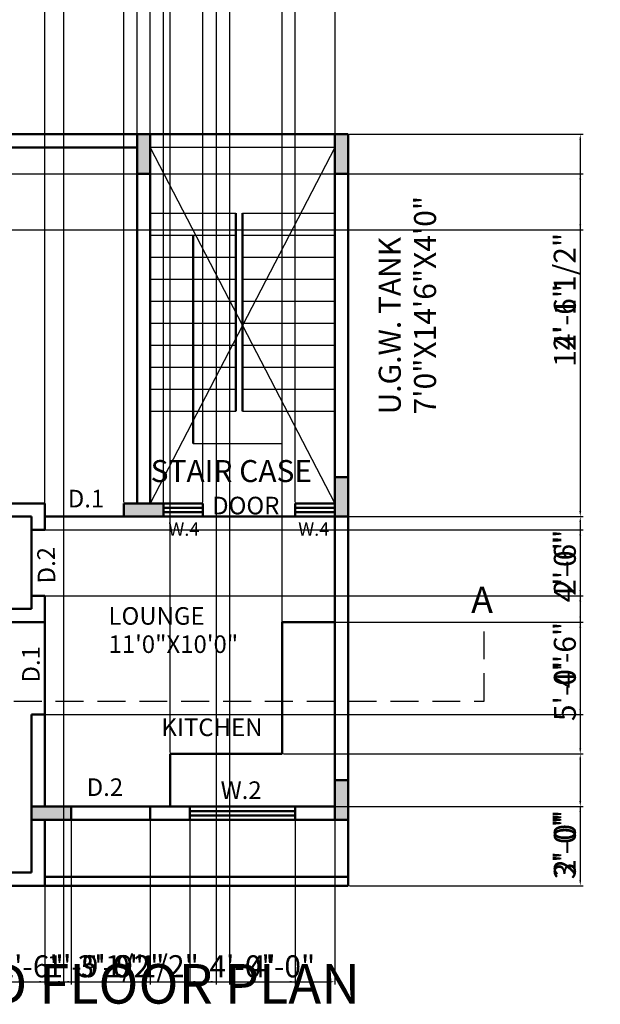
# Model space of a CAD drawing. Units: inches. Extents: x 2368 to 3882, y 1243 to 2139.
# Tile 2 of 6: x 2595 to 2859, y 1243 to 1691. Entities that reach past the tile are written whole.
import ezdxf

# ---------------------------------------------------------------- set-up
doc = ezdxf.new("R2010")
doc.units = ezdxf.units.IN
doc.linetypes.add('DASHED', pattern=[19.05, 12.7, -6.35])
for name, color, linetype, lineweight in [('A-ANNO-DIMS', 2, 'Continuous', 18), ('A-ANNO-SYMB', 1, 'DASHED', 25), ('A-ANNO-TEXT', 7, 'Continuous', 18), ('A-AREA-IDEN', 3, 'Continuous', 18), ('A-FLOR-STRS', 3, 'Continuous', 25), ('A-WALL', 7, 'Continuous', 50), ('A-WALL-PATT', 8, 'Continuous', 13)]:
    doc.layers.add(name, color=color, linetype=linetype, lineweight=lineweight)
doc.styles.get("Standard").update_dxf_attribs({"font": 'arial.ttf'})
doc.dimstyles.new('ISO-25', dxfattribs={"dimtxt": 10, "dimasz": 2.5, "dimexe": 1.25, "dimexo": 0.625, "dimtad": 1, "dimlunit": 3, "dimtxsty": 'Standard', "dimcen": 2.5, "dimadec": 0, "dimazin": 0, "dimtfac": 1, "dimtmove": 0, "dimatfit": 3, "dimfxl": 1, "dimarcsym": 0})

# ---------------------------------------------------------------- blocks, each defined once
blk = doc.blocks.new('*D35')
at = {"layer": 'A-ANNO-DIMS', "color": 0, "lineweight": -2, "transparency": 16777216}
for p, q in [((2585.04, 1776.18), (2585.04, 1251.93)), ((2615.04, 1776.18), (2615.04, 1251.93)), ((2587.54, 1253.18), (2612.54, 1253.18))]:
    blk.add_line(p, q, dxfattribs=at)
at = {"layer": 'A-ANNO-DIMS', "color": 0, "transparency": 16777216}
for points in [[(2587.54, 1253.6), (2587.54, 1252.77), (2585.04, 1253.18)], [(2612.54, 1253.6), (2612.54, 1252.77), (2615.04, 1253.18)]]:
    blk.add_solid(points, dxfattribs=at)
at = {"layer": 'Defpoints', "color": 0, "transparency": 16777216}
for p in [(2585.04, 1776.81), (2615.04, 1776.81), (2615.04, 1253.18)]:
    blk.add_point(p, dxfattribs=at)
at = {"layer": 'A-ANNO-DIMS', "color": 0, "transparency": 16777216, "insert": (2600.04, 1258.91), "char_height": 10, "attachment_point": 5}
blk.add_mtext('2\'-6"', dxfattribs=at)
blk = doc.blocks.new('*D36')
at = {"layer": 'A-ANNO-DIMS', "color": 0, "lineweight": -2, "transparency": 16777216}
for p, q in [((2615.04, 1776.18), (2615.04, 1251.93)), ((2684.5, 1770.18), (2684.5, 1251.93)), ((2617.54, 1253.18), (2682, 1253.18))]:
    blk.add_line(p, q, dxfattribs=at)
at = {"layer": 'A-ANNO-DIMS', "color": 0, "transparency": 16777216}
for points in [[(2617.54, 1253.6), (2617.54, 1252.77), (2615.04, 1253.18)], [(2682, 1253.6), (2682, 1252.77), (2684.5, 1253.18)]]:
    blk.add_solid(points, dxfattribs=at)
at = {"layer": 'Defpoints', "color": 0, "transparency": 16777216}
for p in [(2615.04, 1776.81), (2684.5, 1770.81), (2684.5, 1253.18)]:
    blk.add_point(p, dxfattribs=at)
at = {"layer": 'A-ANNO-DIMS', "color": 0, "transparency": 16777216, "insert": (2649.77, 1258.98), "char_height": 10, "attachment_point": 5}
blk.add_mtext('5\'-9 1/2"', dxfattribs=at)
blk = doc.blocks.new('*D37')
at = {"layer": 'A-ANNO-DIMS', "color": 0, "lineweight": -2, "transparency": 16777216}
for p, q in [((2690.5, 1770.18), (2690.5, 1251.93)), ((2738.5, 1770.18), (2738.5, 1251.93)), ((2693, 1253.18), (2736, 1253.18))]:
    blk.add_line(p, q, dxfattribs=at)
at = {"layer": 'A-ANNO-DIMS', "color": 0, "transparency": 16777216}
for points in [[(2693, 1253.6), (2693, 1252.77), (2690.5, 1253.18)], [(2736, 1253.6), (2736, 1252.77), (2738.5, 1253.18)]]:
    blk.add_solid(points, dxfattribs=at)
at = {"layer": 'Defpoints', "color": 0, "transparency": 16777216}
for p in [(2690.5, 1770.81), (2738.5, 1770.81), (2738.5, 1253.18)]:
    blk.add_point(p, dxfattribs=at)
at = {"layer": 'A-ANNO-DIMS', "color": 0, "transparency": 16777216, "insert": (2714.5, 1258.91), "char_height": 10, "attachment_point": 5}
blk.add_mtext('4\'-0"', dxfattribs=at)
blk = doc.blocks.new('*D45')
at = {"layer": 'A-ANNO-DIMS', "color": 0, "lineweight": -2, "transparency": 16777216}
for p, q in [((2745.12, 1638.88), (2851.45, 1638.88)), ((2850.2, 1636.38), (2850.2, 1467.38)), ((2739.12, 1464.88), (2851.45, 1464.88))]:
    blk.add_line(p, q, dxfattribs=at)
at = {"layer": 'A-ANNO-DIMS', "color": 0, "transparency": 16777216}
for points in [[(2849.79, 1636.38), (2850.62, 1636.38), (2850.2, 1638.88)], [(2849.79, 1467.38), (2850.62, 1467.38), (2850.2, 1464.88)]]:
    blk.add_solid(points, dxfattribs=at)
at = {"layer": 'Defpoints', "color": 0, "transparency": 16777216}
for p in [(2744.5, 1638.88), (2738.5, 1464.88), (2850.2, 1464.88)]:
    blk.add_point(p, dxfattribs=at)
at = {"layer": 'A-ANNO-DIMS', "color": 0, "transparency": 16777216, "insert": (2844.47, 1551.88), "char_height": 10, "attachment_point": 5, "rotation": 90}
blk.add_mtext('14\'-6"', dxfattribs=at)
blk = doc.blocks.new('*D46')
at = {"layer": 'A-ANNO-DIMS', "color": 0, "lineweight": -2, "transparency": 16777216}
for p, q in [((2739.12, 1464.88), (2851.45, 1464.88)), ((2850.2, 1462.38), (2850.2, 1419.38)), ((2715.12, 1416.88), (2851.45, 1416.88))]:
    blk.add_line(p, q, dxfattribs=at)
at = {"layer": 'A-ANNO-DIMS', "color": 0, "transparency": 16777216}
for points in [[(2849.79, 1462.38), (2850.62, 1462.38), (2850.2, 1464.88)], [(2849.79, 1419.38), (2850.62, 1419.38), (2850.2, 1416.88)]]:
    blk.add_solid(points, dxfattribs=at)
at = {"layer": 'Defpoints', "color": 0, "transparency": 16777216}
for p in [(2738.5, 1464.88), (2714.5, 1416.88), (2850.2, 1416.88)]:
    blk.add_point(p, dxfattribs=at)
at = {"layer": 'A-ANNO-DIMS', "color": 0, "transparency": 16777216, "insert": (2844.47, 1440.88), "char_height": 10, "attachment_point": 5, "rotation": 90}
blk.add_mtext('4\'-0"', dxfattribs=at)
blk = doc.blocks.new('*D47')
at = {"layer": 'A-ANNO-DIMS', "color": 0, "lineweight": -2, "transparency": 16777216}
for p, q in [((2715.12, 1416.88), (2851.45, 1416.88)), ((2850.2, 1414.38), (2850.2, 1359.38)), ((2715.12, 1356.88), (2851.45, 1356.88))]:
    blk.add_line(p, q, dxfattribs=at)
at = {"layer": 'A-ANNO-DIMS', "color": 0, "transparency": 16777216}
for points in [[(2849.79, 1414.38), (2850.62, 1414.38), (2850.2, 1416.88)], [(2849.79, 1359.38), (2850.62, 1359.38), (2850.2, 1356.88)]]:
    blk.add_solid(points, dxfattribs=at)
at = {"layer": 'Defpoints', "color": 0, "transparency": 16777216}
for p in [(2714.5, 1416.88), (2714.5, 1356.88), (2850.2, 1356.88)]:
    blk.add_point(p, dxfattribs=at)
at = {"layer": 'A-ANNO-DIMS', "color": 0, "transparency": 16777216, "insert": (2844.47, 1386.88), "char_height": 10, "attachment_point": 5, "rotation": 90}
blk.add_mtext('5\'-0"', dxfattribs=at)
blk = doc.blocks.new('*D48')
at = {"layer": 'A-ANNO-DIMS', "color": 0, "lineweight": -2, "transparency": 16777216}
for p, q in [((2715.12, 1356.88), (2851.45, 1356.88)), ((2850.2, 1354.38), (2850.2, 1335.38)), ((2739.12, 1332.88), (2851.45, 1332.88)), ((2850.2, 1332.88), (2850.2, 1302.38))]:
    blk.add_line(p, q, dxfattribs=at)
at = {"layer": 'A-ANNO-DIMS', "color": 0, "transparency": 16777216}
for points in [[(2849.79, 1354.38), (2850.62, 1354.38), (2850.2, 1356.88)], [(2849.79, 1335.38), (2850.62, 1335.38), (2850.2, 1332.88)]]:
    blk.add_solid(points, dxfattribs=at)
at = {"layer": 'Defpoints', "color": 0, "transparency": 16777216}
for p in [(2714.5, 1356.88), (2738.5, 1332.88), (2850.2, 1332.88)]:
    blk.add_point(p, dxfattribs=at)
at = {"layer": 'A-ANNO-DIMS', "color": 0, "transparency": 16777216, "insert": (2844.47, 1316.38), "char_height": 10, "attachment_point": 5, "rotation": 90}
blk.add_mtext('2\'-0"', dxfattribs=at)
blk = doc.blocks.new('*D49')
at = {"layer": 'A-ANNO-DIMS', "color": 0, "lineweight": -2, "transparency": 16777216}
for p, q in [((2739.12, 1332.88), (2851.45, 1332.88)), ((2850.2, 1330.38), (2850.2, 1299.38)), ((2745.12, 1296.88), (2851.45, 1296.88))]:
    blk.add_line(p, q, dxfattribs=at)
at = {"layer": 'A-ANNO-DIMS', "color": 0, "transparency": 16777216}
for points in [[(2849.79, 1330.38), (2850.62, 1330.38), (2850.2, 1332.88)], [(2849.79, 1299.38), (2850.62, 1299.38), (2850.2, 1296.88)]]:
    blk.add_solid(points, dxfattribs=at)
at = {"layer": 'Defpoints', "color": 0, "transparency": 16777216}
for p in [(2738.5, 1332.88), (2744.5, 1296.88), (2850.2, 1296.88)]:
    blk.add_point(p, dxfattribs=at)
at = {"layer": 'A-ANNO-DIMS', "color": 0, "transparency": 16777216, "insert": (2844.47, 1314.88), "char_height": 10, "attachment_point": 5, "rotation": 90}
blk.add_mtext('3\'-0"', dxfattribs=at)
blk = doc.blocks.new('*D50')
at = {"layer": 'A-ANNO-DIMS', "color": 0, "lineweight": -2, "transparency": 16777216}
for p, q in [((2582.5, 1633.51), (2582.5, 2127.76)), ((2585, 2126.51), (2646, 2126.51)), ((2648.5, 1639.51), (2648.5, 2127.76))]:
    blk.add_line(p, q, dxfattribs=at)
at = {"layer": 'A-ANNO-DIMS', "color": 0, "transparency": 16777216}
for points in [[(2585, 2126.93), (2585, 2126.09), (2582.5, 2126.51)], [(2646, 2126.93), (2646, 2126.09), (2648.5, 2126.51)]]:
    blk.add_solid(points, dxfattribs=at)
at = {"layer": 'Defpoints', "color": 0, "transparency": 16777216}
for p in [(2648.5, 2126.51), (2648.5, 1638.88), (2582.5, 1632.88)]:
    blk.add_point(p, dxfattribs=at)
at = {"layer": 'A-ANNO-DIMS', "color": 0, "transparency": 16777216, "insert": (2615.5, 2132.24), "char_height": 10, "attachment_point": 5}
blk.add_mtext('5\'-6"', dxfattribs=at)
blk = doc.blocks.new('*D51')
at = {"layer": 'A-ANNO-DIMS', "color": 0, "lineweight": -2, "transparency": 16777216}
for p, q in [((2646, 2126.51), (2643.5, 2126.51)), ((2648.5, 1639.51), (2648.5, 2127.76)), ((2648.5, 2126.51), (2654.5, 2126.51)), ((2654.5, 1639.51), (2654.5, 2127.76)), ((2657, 2126.51), (2687.33, 2126.51))]:
    blk.add_line(p, q, dxfattribs=at)
at = {"layer": 'A-ANNO-DIMS', "color": 0, "transparency": 16777216}
for points in [[(2646, 2126.93), (2646, 2126.09), (2648.5, 2126.51)], [(2657, 2126.93), (2657, 2126.09), (2654.5, 2126.51)]]:
    blk.add_solid(points, dxfattribs=at)
at = {"layer": 'Defpoints', "color": 0, "transparency": 16777216}
for p in [(2654.5, 2126.51), (2648.5, 1638.88), (2654.5, 1638.88)]:
    blk.add_point(p, dxfattribs=at)
at = {"layer": 'A-ANNO-DIMS', "color": 0, "transparency": 16777216, "insert": (2673.41, 2132.24), "char_height": 10, "attachment_point": 5}
blk.add_mtext('0\'-6"', dxfattribs=at)
blk = doc.blocks.new('*D53')
at = {"layer": 'A-ANNO-DIMS', "color": 0, "lineweight": -2, "transparency": 16777216}
for p, q in [((2663.5, 1357.51), (2663.5, 2127.76)), ((2666, 2126.51), (2712, 2126.51)), ((2714.5, 1357.51), (2714.5, 2127.76))]:
    blk.add_line(p, q, dxfattribs=at)
at = {"layer": 'A-ANNO-DIMS', "color": 0, "transparency": 16777216}
for points in [[(2666, 2126.93), (2666, 2126.09), (2663.5, 2126.51)], [(2712, 2126.93), (2712, 2126.09), (2714.5, 2126.51)]]:
    blk.add_solid(points, dxfattribs=at)
at = {"layer": 'Defpoints', "color": 0, "transparency": 16777216}
for p in [(2714.5, 2126.51), (2663.5, 1356.88), (2714.5, 1356.88)]:
    blk.add_point(p, dxfattribs=at)
at = {"layer": 'A-ANNO-DIMS', "color": 0, "transparency": 16777216, "insert": (2689, 2132.24), "char_height": 10, "attachment_point": 5}
blk.add_mtext('4\'-3"', dxfattribs=at)
blk = doc.blocks.new('*D55')
at = {"layer": 'A-ANNO-DIMS', "color": 0, "lineweight": -2, "transparency": 16777216}
for p, q in [((2585.04, 1296.26), (2585.04, 1251.93)), ((2606.5, 1296.26), (2606.5, 1251.93)), ((2587.54, 1253.18), (2604, 1253.18)), ((2606.5, 1253.18), (2659.19, 1253.18))]:
    blk.add_line(p, q, dxfattribs=at)
at = {"layer": 'A-ANNO-DIMS', "color": 0, "transparency": 16777216}
for points in [[(2587.54, 1253.6), (2587.54, 1252.77), (2585.04, 1253.18)], [(2604, 1253.6), (2604, 1252.77), (2606.5, 1253.18)]]:
    blk.add_solid(points, dxfattribs=at)
at = {"layer": 'Defpoints', "color": 0, "transparency": 16777216}
for p in [(2585.04, 1296.88), (2606.5, 1296.88), (2606.5, 1253.18)]:
    blk.add_point(p, dxfattribs=at)
at = {"layer": 'A-ANNO-DIMS', "color": 0, "transparency": 16777216, "insert": (2634.09, 1258.98), "char_height": 10, "attachment_point": 5}
blk.add_mtext('1\'-9 1/2"', dxfattribs=at)
blk = doc.blocks.new('*D56')
at = {"layer": 'A-ANNO-DIMS', "color": 0, "lineweight": -2, "transparency": 16777216}
for p, q in [((2618.5, 1332.26), (2618.5, 1251.93)), ((2654.5, 1332.26), (2654.5, 1251.93)), ((2621, 1253.18), (2652, 1253.18))]:
    blk.add_line(p, q, dxfattribs=at)
at = {"layer": 'A-ANNO-DIMS', "color": 0, "transparency": 16777216}
for points in [[(2621, 1253.6), (2621, 1252.77), (2618.5, 1253.18)], [(2652, 1253.6), (2652, 1252.77), (2654.5, 1253.18)]]:
    blk.add_solid(points, dxfattribs=at)
at = {"layer": 'Defpoints', "color": 0, "transparency": 16777216}
for p in [(2618.5, 1332.88), (2654.5, 1332.88), (2654.5, 1253.18)]:
    blk.add_point(p, dxfattribs=at)
at = {"layer": 'A-ANNO-DIMS', "color": 0, "transparency": 16777216, "insert": (2636.5, 1258.92), "char_height": 10, "attachment_point": 5}
blk.add_mtext('3\'-0"', dxfattribs=at)
blk = doc.blocks.new('*D57')
at = {"layer": 'A-ANNO-DIMS', "color": 0, "lineweight": -2, "transparency": 16777216}
for p, q in [((2672.5, 1326.26), (2672.5, 1251.93)), ((2720.5, 1326.26), (2720.5, 1251.93)), ((2675, 1253.18), (2718, 1253.18))]:
    blk.add_line(p, q, dxfattribs=at)
at = {"layer": 'A-ANNO-DIMS', "color": 0, "transparency": 16777216}
for points in [[(2675, 1253.6), (2675, 1252.77), (2672.5, 1253.18)], [(2718, 1253.6), (2718, 1252.77), (2720.5, 1253.18)]]:
    blk.add_solid(points, dxfattribs=at)
at = {"layer": 'Defpoints', "color": 0, "transparency": 16777216}
for p in [(2672.5, 1326.88), (2720.5, 1326.88), (2720.5, 1253.18)]:
    blk.add_point(p, dxfattribs=at)
at = {"layer": 'A-ANNO-DIMS', "color": 0, "transparency": 16777216, "insert": (2696.5, 1258.91), "char_height": 10, "attachment_point": 5}
blk.add_mtext('4\'-0"', dxfattribs=at)
blk = doc.blocks.new('*D59')
at = {"layer": 'A-ANNO-DIMS', "color": 0, "lineweight": -2, "transparency": 16777216}
for p, q in [((2606.5, 1465.51), (2606.5, 2127.76)), ((2609, 2126.51), (2640, 2126.51)), ((2642.5, 1471.51), (2642.5, 2127.76))]:
    blk.add_line(p, q, dxfattribs=at)
at = {"layer": 'A-ANNO-DIMS', "color": 0, "transparency": 16777216}
for points in [[(2609, 2126.93), (2609, 2126.09), (2606.5, 2126.51)], [(2640, 2126.93), (2640, 2126.09), (2642.5, 2126.51)]]:
    blk.add_solid(points, dxfattribs=at)
at = {"layer": 'Defpoints', "color": 0, "transparency": 16777216}
for p in [(2642.5, 2126.51), (2642.5, 1470.88), (2606.5, 1464.88)]:
    blk.add_point(p, dxfattribs=at)
at = {"layer": 'A-ANNO-DIMS', "color": 0, "transparency": 16777216, "insert": (2624.5, 2132.24), "char_height": 10, "attachment_point": 5}
blk.add_mtext('3\'-0"', dxfattribs=at)
blk = doc.blocks.new('*D60')
at = {"layer": 'A-ANNO-DIMS', "color": 0, "lineweight": -2, "transparency": 16777216}
for p, q in [((2660.5, 1471.51), (2660.5, 2127.76)), ((2663, 2126.51), (2676, 2126.51)), ((2678.5, 1471.51), (2678.5, 2127.76)), ((2678.5, 2126.51), (2707.89, 2126.51))]:
    blk.add_line(p, q, dxfattribs=at)
at = {"layer": 'A-ANNO-DIMS', "color": 0, "transparency": 16777216}
for points in [[(2663, 2126.93), (2663, 2126.09), (2660.5, 2126.51)], [(2676, 2126.93), (2676, 2126.09), (2678.5, 2126.51)]]:
    blk.add_solid(points, dxfattribs=at)
at = {"layer": 'Defpoints', "color": 0, "transparency": 16777216}
for p in [(2678.5, 2126.51), (2660.5, 1470.88), (2678.5, 1470.88)]:
    blk.add_point(p, dxfattribs=at)
at = {"layer": 'A-ANNO-DIMS', "color": 0, "transparency": 16777216, "insert": (2694.44, 2132.24), "char_height": 10, "attachment_point": 5}
blk.add_mtext('1\'-6"', dxfattribs=at)
blk = doc.blocks.new('*D61')
at = {"layer": 'A-ANNO-DIMS', "color": 0, "lineweight": -2, "transparency": 16777216}
for p, q in [((2678.5, 1471.51), (2678.5, 2127.76)), ((2681, 2126.51), (2718, 2126.51)), ((2720.5, 1471.51), (2720.5, 2127.76))]:
    blk.add_line(p, q, dxfattribs=at)
at = {"layer": 'A-ANNO-DIMS', "color": 0, "transparency": 16777216}
for points in [[(2681, 2126.93), (2681, 2126.09), (2678.5, 2126.51)], [(2718, 2126.93), (2718, 2126.09), (2720.5, 2126.51)]]:
    blk.add_solid(points, dxfattribs=at)
at = {"layer": 'Defpoints', "color": 0, "transparency": 16777216}
for p in [(2720.5, 2126.51), (2678.5, 1470.88), (2720.5, 1470.88)]:
    blk.add_point(p, dxfattribs=at)
at = {"layer": 'A-ANNO-DIMS', "color": 0, "transparency": 16777216, "insert": (2699.5, 2132.24), "char_height": 10, "attachment_point": 5}
blk.add_mtext('3\'-6"', dxfattribs=at)
blk = doc.blocks.new('*D63')
at = {"layer": 'A-ANNO-DIMS', "color": 0, "lineweight": -2, "transparency": 16777216}
for p, q in [((2577.12, 1620.88), (2851.45, 1620.88)), ((2850.2, 1618.38), (2850.2, 1597.8)), ((2577.12, 1595.3), (2851.45, 1595.3)), ((2850.2, 1595.3), (2850.2, 1541.5))]:
    blk.add_line(p, q, dxfattribs=at)
at = {"layer": 'A-ANNO-DIMS', "color": 0, "transparency": 16777216}
for points in [[(2849.79, 1618.38), (2850.62, 1618.38), (2850.2, 1620.88)], [(2849.79, 1597.8), (2850.62, 1597.8), (2850.2, 1595.3)]]:
    blk.add_solid(points, dxfattribs=at)
at = {"layer": 'Defpoints', "color": 0, "transparency": 16777216}
for p in [(2576.5, 1620.88), (2576.5, 1595.3), (2850.2, 1595.3)]:
    blk.add_point(p, dxfattribs=at)
at = {"layer": 'A-ANNO-DIMS', "color": 0, "transparency": 16777216, "insert": (2844.41, 1567.15), "char_height": 10, "attachment_point": 5, "rotation": 90}
blk.add_mtext('2\'-1 1/2"', dxfattribs=at)
blk = doc.blocks.new('*D64')
at = {"layer": 'A-ANNO-DIMS', "color": 0, "lineweight": -2, "transparency": 16777216}
for p, q in [((2601.12, 1458.88), (2851.45, 1458.88)), ((2850.2, 1456.38), (2850.2, 1431.38)), ((2601.12, 1428.88), (2851.45, 1428.88))]:
    blk.add_line(p, q, dxfattribs=at)
at = {"layer": 'A-ANNO-DIMS', "color": 0, "transparency": 16777216}
for points in [[(2849.79, 1456.38), (2850.62, 1456.38), (2850.2, 1458.88)], [(2849.79, 1431.38), (2850.62, 1431.38), (2850.2, 1428.88)]]:
    blk.add_solid(points, dxfattribs=at)
at = {"layer": 'Defpoints', "color": 0, "transparency": 16777216}
for p in [(2600.5, 1458.88), (2600.5, 1428.88), (2850.2, 1428.88)]:
    blk.add_point(p, dxfattribs=at)
at = {"layer": 'A-ANNO-DIMS', "color": 0, "transparency": 16777216, "insert": (2844.47, 1443.88), "char_height": 10, "attachment_point": 5, "rotation": 90}
blk.add_mtext('2\'-6"', dxfattribs=at)
blk = doc.blocks.new('*D65')
at = {"layer": 'A-ANNO-DIMS', "color": 0, "lineweight": -2, "transparency": 16777216}
for p, q in [((2607.12, 1428.88), (2851.45, 1428.88)), ((2850.2, 1426.38), (2850.2, 1377.38)), ((2607.12, 1374.88), (2851.45, 1374.88))]:
    blk.add_line(p, q, dxfattribs=at)
at = {"layer": 'A-ANNO-DIMS', "color": 0, "transparency": 16777216}
for points in [[(2849.79, 1426.38), (2850.62, 1426.38), (2850.2, 1428.88)], [(2849.79, 1377.38), (2850.62, 1377.38), (2850.2, 1374.88)]]:
    blk.add_solid(points, dxfattribs=at)
at = {"layer": 'Defpoints', "color": 0, "transparency": 16777216}
for p in [(2606.5, 1428.88), (2606.5, 1374.88), (2850.2, 1374.88)]:
    blk.add_point(p, dxfattribs=at)
at = {"layer": 'A-ANNO-DIMS', "color": 0, "transparency": 16777216, "insert": (2844.47, 1401.88), "char_height": 10, "attachment_point": 5, "rotation": 90}
blk.add_mtext('4\'-6"', dxfattribs=at)

msp = doc.modelspace()

# ---------------------------------------------------------------- hatches: boundary and pattern name
at = {"layer": 'A-WALL-PATT'}
h = msp.add_hatch(color=256, dxfattribs=at)
h.dxf.hatch_style = 1
h.paths.add_polyline_path([(2492.497, 1344.883), (2486.497, 1344.883), (2486.497, 1326.883), (2492.497, 1326.883)])
h.paths.add_polyline_path([(2618.497, 1332.883), (2600.497, 1332.883), (2600.497, 1326.883), (2618.497, 1326.883)])
h.paths.add_polyline_path([(2744.497, 1344.883), (2738.497, 1344.883), (2738.497, 1326.883), (2744.497, 1326.883)])
h.paths.add_polyline_path([(2744.497, 1482.883), (2738.497, 1482.883), (2738.497, 1464.883), (2744.497, 1464.883)])
h.paths.add_polyline_path([(2660.497, 1470.883), (2642.497, 1470.883), (2642.497, 1464.883), (2660.497, 1464.883)])
h.paths.add_polyline_path([(2492.497, 1482.883), (2486.497, 1482.883), (2486.497, 1464.883), (2492.497, 1464.883)])
h.paths.add_polyline_path([(2492.497, 1638.883), (2486.497, 1638.883), (2486.497, 1620.883), (2492.497, 1620.883)])
h.paths.add_polyline_path([(2654.497, 1638.883), (2648.497, 1638.883), (2648.497, 1620.883), (2654.497, 1620.883)])
h.paths.add_polyline_path([(2744.497, 1638.883), (2738.497, 1638.883), (2738.497, 1620.883), (2744.497, 1620.883)])
h.paths.add_polyline_path([(2744.497, 1788.809), (2738.497, 1788.809), (2738.497, 1770.809), (2744.497, 1770.809)])
h.paths.add_polyline_path([(2615.041, 1776.809), (2597.041, 1776.809), (2597.041, 1770.809), (2615.041, 1770.809)])
h.paths.add_polyline_path([(2492.497, 1788.809), (2486.497, 1788.809), (2486.497, 1770.809), (2492.497, 1770.809)])
h.paths.add_polyline_path([(2492.497, 1926.809), (2486.497, 1926.809), (2486.497, 1908.809), (2492.497, 1908.809)])
h.paths.add_polyline_path([(2660.497, 1914.809), (2642.497, 1914.809), (2642.497, 1908.809), (2660.497, 1908.809)])
h.paths.add_polyline_path([(2744.497, 1926.809), (2738.497, 1926.809), (2738.497, 1908.809), (2744.497, 1908.809)])
h.paths.add_polyline_path([(2744.497, 2082.809), (2738.497, 2082.809), (2738.497, 2064.809), (2744.497, 2064.809)])
h.paths.add_polyline_path([(2654.497, 2082.809), (2648.497, 2082.809), (2648.497, 2064.809), (2654.497, 2064.809)])
h.paths.add_polyline_path([(2492.497, 2082.809), (2486.497, 2082.809), (2486.497, 2064.809), (2492.497, 2064.809)])

# ---------------------------------------------------------------- linework, layer by layer
at = {"layer": 'A-ANNO-SYMB'}
for p, q in [((2806.503, 1380.883), (2806.503, 1417.69)), ((2440.007, 1380.883), (2806.503, 1380.883))]:
    msp.add_line(p, q, dxfattribs=at)
at = {"layer": 'A-FLOR-STRS'}
for p, q in [((2738.497, 1632.883), (2654.497, 1632.883)), ((2738.497, 1632.883), (2654.497, 1470.883)), ((2654.497, 1632.883), (2738.497, 1470.883)), ((2654.497, 1602.883), (2693.497, 1602.883)), ((2696.497, 1602.883), (2738.497, 1602.883)), ((2654.497, 1592.883), (2693.497, 1592.883)), ((2696.497, 1592.883), (2738.497, 1592.883)), ((2654.497, 1582.883), (2693.497, 1582.883)), ((2696.497, 1582.883), (2738.497, 1582.883)), ((2654.497, 1572.883), (2693.497, 1572.883)), ((2696.497, 1572.883), (2738.497, 1572.883)), ((2654.497, 1562.883), (2693.497, 1562.883)), ((2696.497, 1562.883), (2738.497, 1562.883)), ((2714.494, 1498.194), (2714.494, 1562.883)), ((2654.497, 1552.883), (2693.497, 1552.883)), ((2696.497, 1552.883), (2738.497, 1552.883)), ((2654.497, 1542.883), (2693.497, 1542.883)), ((2696.497, 1542.883), (2738.497, 1542.883)), ((2654.497, 1532.883), (2693.497, 1532.883)), ((2696.497, 1532.883), (2738.497, 1532.883)), ((2654.497, 1522.883), (2693.497, 1522.883)), ((2696.497, 1522.883), (2738.497, 1522.883)), ((2654.497, 1512.883), (2693.497, 1512.883)), ((2696.497, 1512.883), (2738.497, 1512.883)), ((2673.997, 1498.194), (2714.494, 1498.194))]:
    msp.add_line(p, q, dxfattribs=at)
at = {"layer": 'A-WALL'}
for p, q in [((2744.497, 1638.883), (2486.497, 1638.883)), ((2648.497, 1470.883), (2648.497, 1638.883)), ((2654.497, 1470.883), (2654.497, 1638.883)), ((2738.497, 1326.883), (2738.497, 1638.883)), ((2744.497, 1296.883), (2744.497, 1638.883)), ((2648.497, 1632.883), (2582.497, 1632.883)), ((2654.497, 1620.883), (2648.497, 1620.883)), ((2744.497, 1620.883), (2738.497, 1620.883)), ((2693.497, 1512.883), (2693.497, 1602.883)), ((2696.497, 1512.883), (2696.497, 1602.883)), ((2673.997, 1592.883), (2673.997, 1498.194)), ((2744.497, 1482.883), (2738.497, 1482.883)), ((2492.497, 1470.883), (2606.497, 1470.883)), ((2606.497, 1470.883), (2606.497, 1458.883)), ((2642.497, 1470.883), (2678.497, 1470.883)), ((2642.497, 1470.883), (2642.497, 1464.883)), ((2660.497, 1470.883), (2660.497, 1464.883)), ((2678.497, 1464.883), (2678.497, 1470.883)), ((2720.497, 1464.883), (2720.497, 1470.883)), ((2720.497, 1470.883), (2738.497, 1470.883)), ((2678.497, 1468.883), (2660.497, 1468.883)), ((2660.497, 1466.883), (2678.497, 1466.883)), ((2738.497, 1468.883), (2720.497, 1468.883)), ((2720.497, 1466.883), (2738.497, 1466.883)), ((2558.497, 1464.883), (2600.497, 1464.883)), ((2600.497, 1464.883), (2600.497, 1422.883)), ((2606.497, 1464.883), (2684.497, 1464.883)), ((2684.497, 1464.883), (2738.497, 1464.883)), ((2744.497, 1464.883), (2738.497, 1464.883)), ((2600.497, 1458.883), (2606.497, 1458.883)), ((2600.497, 1428.883), (2606.497, 1428.883)), ((2606.497, 1428.883), (2606.497, 1332.883)), ((2558.497, 1422.883), (2600.497, 1422.883)), ((2591.497, 1416.883), (2606.497, 1416.883)), ((2714.497, 1356.883), (2714.497, 1416.883)), ((2714.497, 1416.883), (2738.497, 1416.883)), ((2600.497, 1374.883), (2600.497, 1302.883)), ((2606.497, 1374.883), (2600.497, 1374.883)), ((2663.497, 1332.883), (2663.497, 1356.883)), ((2663.497, 1356.883), (2714.497, 1356.883)), ((2744.497, 1344.883), (2738.497, 1344.883)), ((2600.497, 1332.883), (2738.497, 1332.883)), ((2618.497, 1326.883), (2618.497, 1332.883)), ((2654.497, 1326.883), (2654.497, 1332.883)), ((2672.497, 1326.883), (2672.497, 1332.883)), ((2672.497, 1330.883), (2720.497, 1330.883)), ((2720.497, 1326.883), (2720.497, 1332.883)), ((2600.497, 1326.883), (2744.497, 1326.883)), ((2606.497, 1326.883), (2606.497, 1302.883)), ((2720.497, 1328.883), (2672.497, 1328.883)), ((2492.497, 1302.883), (2600.497, 1302.883)), ((2606.497, 1302.883), (2606.497, 1296.883)), ((2606.497, 1300.883), (2744.497, 1300.883)), ((2486.497, 1296.883), (2744.497, 1296.883))]:
    msp.add_line(p, q, dxfattribs=at)

# ---------------------------------------------------------------- texts
at = {"layer": 'A-ANNO-SYMB'}
msp.add_text('A', height=12, dxfattribs=at).set_placement((2800.512, 1420.988))
at = {"layer": 'A-ANNO-TEXT'}
for s, height, p in [('D.1', 8, (2616.968, 1469.05)), ('DOOR', 8, (2682.656, 1465.89)), ('D.2', 8, (2625.573, 1337.734)), ('W.2', 8, (2686.528, 1336.372)), ('1ST TO 3RD FLOOR PLAN', 18, (2465.517, 1243.248))]:
    msp.add_text(s, height=height, dxfattribs=at).set_placement(p)
for s, height, rotation, p in [('W.4', 6.0503, 0.00222, (2662.746, 1456.14)), ('W.4', 6.0503, 0.00222, (2721.847, 1456.14)), ('D.2', 8, 91.16562, (2611.355, 1434.518)), ('D.1', 8, 90, (2604.191, 1389.36))]:
    msp.add_text(s, height=height, rotation=rotation, dxfattribs=at).set_placement(p)
at = {"layer": 'A-AREA-IDEN'}
for s, p in [('7\'0"X14\'6"X4\'0"', (2784.562, 1511.375)), ('U.G.W. TANK', (2768.498, 1511.375))]:
    msp.add_text(s, height=10, rotation=90, dxfattribs=at).set_placement(p)
for s, height, p in [('STAIR CASE', 10, (2654.672, 1480.599)), ('LOUNGE', 8, (2635.498, 1415.658)), ('11\'0"X10\'0"', 8, (2635.498, 1402.807)), ('KITCHEN', 8, (2659.574, 1364.991))]:
    msp.add_text(s, height=height, dxfattribs=at).set_placement(p)

# ---------------------------------------------------------------- dimensions: what is measured, and where the dimension line sits
at = {"layer": 'A-ANNO-DIMS'}
for base, p1, p2, picture, middle in [((2648.497, 2126.509), (2582.497, 1632.883), (2648.497, 1638.883), '*D50', (2615.497, 2132.24)), ((2642.497, 2126.509), (2606.497, 1464.883), (2642.497, 1470.883), '*D59', (2624.497, 2132.243)), ((2654.497, 2126.509), (2648.497, 1638.883), (2654.497, 1638.883), '*D51', (2673.414, 2132.24)), ((2678.497, 2126.509), (2660.497, 1470.883), (2678.497, 1470.883), '*D60', (2694.443, 2132.24)), ((2714.497, 2126.509), (2663.497, 1356.883), (2714.497, 1356.883), '*D53', (2688.997, 2132.243)), ((2720.497, 2126.509), (2678.497, 1470.883), (2720.497, 1470.883), '*D61', (2699.497, 2132.243)), ((2615.041, 1253.183), (2585.041, 1776.809), (2615.041, 1776.809), '*D35', (2600.041, 1258.914)), ((2684.497, 1253.183), (2615.041, 1776.809), (2684.497, 1770.809), '*D36', (2649.769, 1258.979)), ((2738.497, 1253.183), (2690.497, 1770.809), (2738.497, 1770.809), '*D37', (2714.497, 1258.914)), ((2654.497, 1253.183), (2618.497, 1332.883), (2654.497, 1332.883), '*D56', (2636.497, 1258.917)), ((2720.497, 1253.183), (2672.497, 1326.883), (2720.497, 1326.883), '*D57', (2696.497, 1258.914)), ((2606.497, 1253.183), (2585.041, 1296.883), (2606.497, 1296.883), '*D55', (2634.094, 1258.979))]:
    dim = msp.add_linear_dim(base=base, p1=p1, p2=p2, dimstyle='ISO-25', override={"dimdec": 1, "dimlfac": 1, "dimrnd": 0, "dimzin": 1, "dimdsep": 46, "dimlunit": 4, "dimfrac": 2}, dxfattribs=at)
    dim.commit()
    dim.dimension.update_dxf_attribs({"geometry": picture, "text_midpoint": middle})
for base, p1, p2, picture, middle in [((2850.203, 1464.883), (2744.497, 1638.883), (2738.497, 1464.883), '*D45', (2844.472, 1551.883)), ((2850.203, 1595.303), (2576.497, 1620.883), (2576.497, 1595.303), '*D63', (2844.408, 1567.15)), ((2850.203, 1416.883), (2738.497, 1464.883), (2714.497, 1416.883), '*D46', (2844.472, 1440.883)), ((2850.203, 1428.883), (2600.497, 1458.883), (2600.497, 1428.883), '*D64', (2844.472, 1443.883)), ((2850.203, 1374.883), (2606.497, 1428.883), (2606.497, 1374.883), '*D65', (2844.472, 1401.883)), ((2850.203, 1356.883), (2714.497, 1416.883), (2714.497, 1356.883), '*D47', (2844.472, 1386.883)), ((2850.203, 1332.883), (2714.497, 1356.883), (2738.497, 1332.883), '*D48', (2844.472, 1316.382)), ((2850.203, 1296.883), (2738.497, 1332.883), (2744.497, 1296.883), '*D49', (2844.469, 1314.883))]:
    dim = msp.add_linear_dim(base=base, p1=p1, p2=p2, angle=90, dimstyle='ISO-25', override={"dimdec": 1, "dimlfac": 1, "dimrnd": 0, "dimzin": 1, "dimdsep": 46, "dimlunit": 4, "dimfrac": 2}, dxfattribs=at)
    dim.commit()
    dim.dimension.update_dxf_attribs({"geometry": picture, "text_midpoint": middle})

doc.saveas('drawing.dxf')
